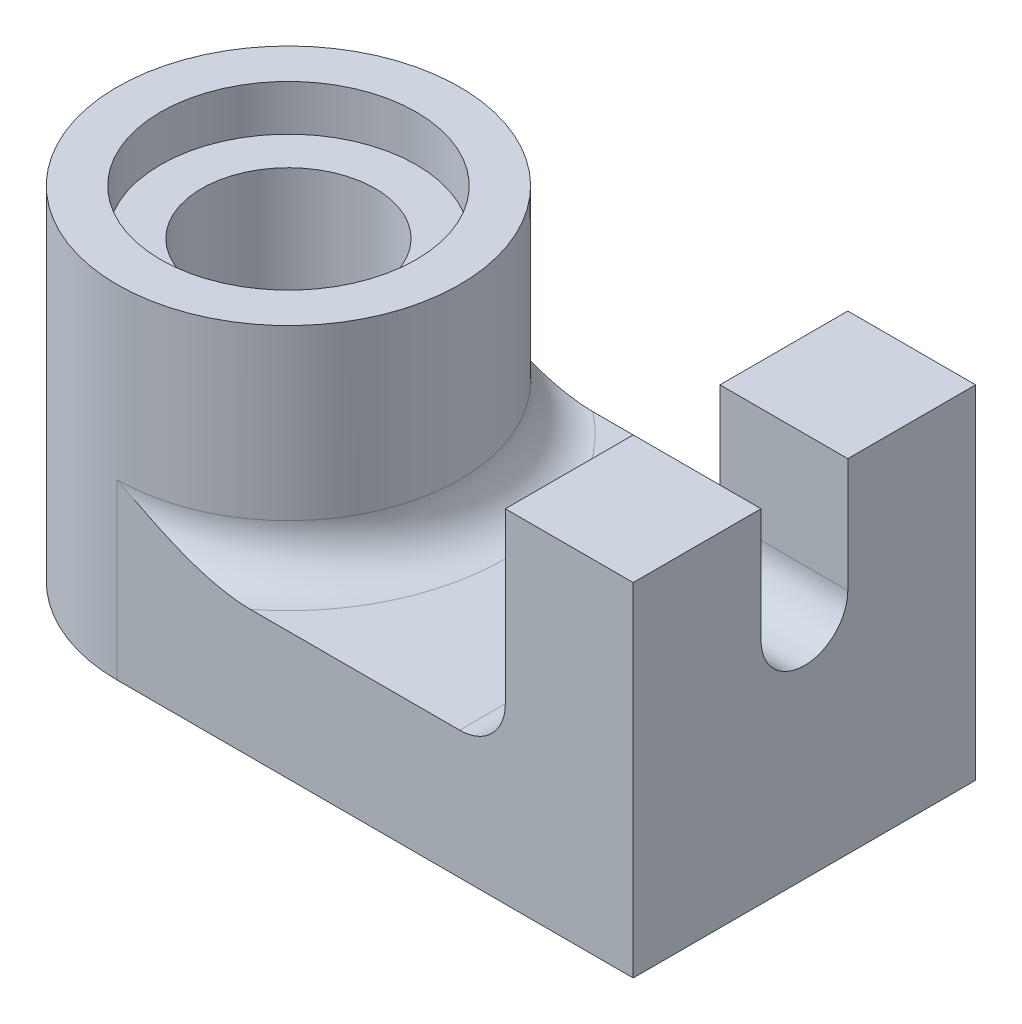
ISO-10303-21;
HEADER;
FILE_DESCRIPTION(('STEP AP214'),'2;1');
FILE_NAME('part.step','',(''),(''),'','','');
FILE_SCHEMA(('AUTOMOTIVE_DESIGN { 1 0 10303 214 1 1 1 1 }'));
ENDSEC;
DATA;
#1=APPLICATION_CONTEXT('core data for automotive mechanical design processes');
#2=APPLICATION_PROTOCOL_DEFINITION('international standard','automotive_design',2000,#1);
#3=PRODUCT_CONTEXT('',#1,'mechanical');
#4=PRODUCT('Part','Part','',(#3));
#5=PRODUCT_RELATED_PRODUCT_CATEGORY('part','',(#4));
#6=PRODUCT_DEFINITION_FORMATION('','',#4);
#7=PRODUCT_DEFINITION_CONTEXT('part definition',#1,'design');
#8=PRODUCT_DEFINITION('design','',#6,#7);
#9=PRODUCT_DEFINITION_SHAPE('','',#8);
#10=(LENGTH_UNIT() NAMED_UNIT(*) SI_UNIT(.MILLI.,.METRE.));
#11=(NAMED_UNIT(*) PLANE_ANGLE_UNIT() SI_UNIT($,.RADIAN.));
#12=(NAMED_UNIT(*) SI_UNIT($,.STERADIAN.) SOLID_ANGLE_UNIT());
#13=UNCERTAINTY_MEASURE_WITH_UNIT(LENGTH_MEASURE(1.E-05),#10,'distance_accuracy_value','');
#14=(GEOMETRIC_REPRESENTATION_CONTEXT(3) GLOBAL_UNCERTAINTY_ASSIGNED_CONTEXT((#13)) GLOBAL_UNIT_ASSIGNED_CONTEXT((#10,
#11,#12)) REPRESENTATION_CONTEXT('',''));
#15=CARTESIAN_POINT('',(0.,0.,0.));
#16=DIRECTION('',(0.,0.,1.));
#17=DIRECTION('',(1.,0.,0.));
#18=AXIS2_PLACEMENT_3D('',#15,#16,#17);
#19=CARTESIAN_POINT('',(0.,75.,0.));
#20=DIRECTION('',(0.,-1.,0.));
#21=DIRECTION('',(0.,0.,-1.));
#22=AXIS2_PLACEMENT_3D('',#19,#20,#21);
#23=PLANE('',#22);
#24=DIRECTION('',(0.,0.,-1.));
#25=VECTOR('',#24,1.);
#26=CARTESIAN_POINT('',(113.,75.,-37.5));
#27=LINE('',#26,#25);
#28=CARTESIAN_POINT('',(113.,75.,37.5));
#29=VERTEX_POINT('',#28);
#30=CARTESIAN_POINT('',(113.,75.,9.49999999999999));
#31=VERTEX_POINT('',#30);
#32=EDGE_CURVE('E204',#29,#31,#27,.T.);
#33=ORIENTED_EDGE('',*,*,#32,.T.);
#34=DIRECTION('',(-1.,0.,0.));
#35=VECTOR('',#34,1.);
#36=CARTESIAN_POINT('',(0.,75.,9.49999999999999));
#37=LINE('',#36,#35);
#38=CARTESIAN_POINT('',(85.,75.,9.49999999999999));
#39=VERTEX_POINT('',#38);
#40=EDGE_CURVE('E267',#31,#39,#37,.T.);
#41=ORIENTED_EDGE('',*,*,#40,.T.);
#42=DIRECTION('',(0.,0.,1.));
#43=VECTOR('',#42,1.);
#44=CARTESIAN_POINT('',(85.,75.,37.5));
#45=LINE('',#44,#43);
#46=CARTESIAN_POINT('',(85.,75.,37.5));
#47=VERTEX_POINT('',#46);
#48=EDGE_CURVE('E207',#39,#47,#45,.T.);
#49=ORIENTED_EDGE('',*,*,#48,.T.);
#50=DIRECTION('',(1.,0.,0.));
#51=VECTOR('',#50,1.);
#52=CARTESIAN_POINT('',(113.,75.,37.5));
#53=LINE('',#52,#51);
#54=EDGE_CURVE('E213',#47,#29,#53,.T.);
#55=ORIENTED_EDGE('',*,*,#54,.T.);
#56=EDGE_LOOP('',(#33,#41,#49,#55));
#57=FACE_BOUND('',#56,.T.);
#58=ADVANCED_FACE('F44',(#57),#23,.F.);
#59=CARTESIAN_POINT('',(0.,28.,0.));
#60=DIRECTION('',(0.,-1.,0.));
#61=DIRECTION('',(0.,0.,-1.));
#62=AXIS2_PLACEMENT_3D('',#59,#60,#61);
#63=PLANE('',#62);
#64=DIRECTION('',(-1.,0.,0.));
#65=VECTOR('',#64,1.);
#66=CARTESIAN_POINT('',(0.,28.,37.5));
#67=LINE('',#66,#65);
#68=CARTESIAN_POINT('',(75.,28.,37.5));
#69=VERTEX_POINT('',#68);
#70=CARTESIAN_POINT('',(29.1547594742265,28.,37.5));
#71=VERTEX_POINT('',#70);
#72=EDGE_CURVE('E223',#69,#71,#67,.T.);
#73=ORIENTED_EDGE('',*,*,#72,.F.);
#74=DIRECTION('',(0.,0.,1.));
#75=VECTOR('',#74,1.);
#76=CARTESIAN_POINT('',(75.,28.,-37.5));
#77=LINE('',#76,#75);
#78=CARTESIAN_POINT('',(75.,28.,-37.5));
#79=VERTEX_POINT('',#78);
#80=EDGE_CURVE('E386',#69,#79,#77,.F.);
#81=ORIENTED_EDGE('',*,*,#80,.T.);
#82=DIRECTION('',(1.,0.,0.));
#83=VECTOR('',#82,1.);
#84=CARTESIAN_POINT('',(113.,28.,-37.5));
#85=LINE('',#84,#83);
#86=CARTESIAN_POINT('',(29.1547594742265,28.,-37.5));
#87=VERTEX_POINT('',#86);
#88=EDGE_CURVE('E225',#87,#79,#85,.T.);
#89=ORIENTED_EDGE('',*,*,#88,.F.);
#90=CARTESIAN_POINT('',(0.,28.,0.));
#91=DIRECTION('',(0.,-1.,0.));
#92=DIRECTION('',(0.,0.,-1.));
#93=AXIS2_PLACEMENT_3D('',#90,#91,#92);
#94=CIRCLE('',#93,47.5);
#95=EDGE_CURVE('E279',#87,#71,#94,.T.);
#96=ORIENTED_EDGE('',*,*,#95,.T.);
#97=EDGE_LOOP('',(#73,#81,#89,#96));
#98=FACE_BOUND('',#97,.T.);
#99=ADVANCED_FACE('F309',(#98),#63,.F.);
#100=CARTESIAN_POINT('',(0.,75.,0.));
#101=DIRECTION('',(0.,-1.,0.));
#102=DIRECTION('',(0.,0.,-1.));
#103=AXIS2_PLACEMENT_3D('',#100,#101,#102);
#104=CYLINDRICAL_SURFACE('',#103,37.5);
#105=CARTESIAN_POINT('',(0.,75.,0.));
#106=DIRECTION('',(0.,1.,0.));
#107=DIRECTION('',(0.,0.,1.));
#108=AXIS2_PLACEMENT_3D('',#105,#106,#107);
#109=CIRCLE('',#108,37.5);
#110=CARTESIAN_POINT('',(0.,75.,37.5));
#111=VERTEX_POINT('',#110);
#112=EDGE_CURVE('E261',#111,#111,#109,.T.);
#113=ORIENTED_EDGE('',*,*,#112,.F.);
#114=EDGE_LOOP('',(#113));
#115=FACE_BOUND('',#114,.T.);
#116=CARTESIAN_POINT('',(0.,38.,0.));
#117=DIRECTION('',(0.,-1.,0.));
#118=DIRECTION('',(0.,0.,-1.));
#119=AXIS2_PLACEMENT_3D('',#116,#117,#118);
#120=CIRCLE('',#119,37.5);
#121=CARTESIAN_POINT('',(0.,38.,37.5));
#122=VERTEX_POINT('',#121);
#123=CARTESIAN_POINT('',(0.,38.,-37.5));
#124=VERTEX_POINT('',#123);
#125=EDGE_CURVE('E274',#122,#124,#120,.F.);
#126=ORIENTED_EDGE('',*,*,#125,.T.);
#127=DIRECTION('',(0.,-1.,0.));
#128=VECTOR('',#127,1.);
#129=CARTESIAN_POINT('',(0.,28.,-37.5));
#130=LINE('',#129,#128);
#131=CARTESIAN_POINT('',(0.,0.,-37.5));
#132=VERTEX_POINT('',#131);
#133=EDGE_CURVE('E230',#124,#132,#130,.T.);
#134=ORIENTED_EDGE('',*,*,#133,.T.);
#135=CARTESIAN_POINT('',(0.,0.,0.));
#136=DIRECTION('',(0.,1.,0.));
#137=DIRECTION('',(0.,0.,1.));
#138=AXIS2_PLACEMENT_3D('',#135,#136,#137);
#139=CIRCLE('',#138,37.5);
#140=CARTESIAN_POINT('',(0.,0.,37.5));
#141=VERTEX_POINT('',#140);
#142=EDGE_CURVE('E256',#132,#141,#139,.T.);
#143=ORIENTED_EDGE('',*,*,#142,.T.);
#144=DIRECTION('',(0.,-1.,0.));
#145=VECTOR('',#144,1.);
#146=CARTESIAN_POINT('',(0.,28.,37.5));
#147=LINE('',#146,#145);
#148=EDGE_CURVE('E237',#122,#141,#147,.T.);
#149=ORIENTED_EDGE('',*,*,#148,.F.);
#150=EDGE_LOOP('',(#126,#134,#143,#149));
#151=FACE_BOUND('',#150,.T.);
#152=ADVANCED_FACE('F304',(#115,#151),#104,.T.);
#153=CARTESIAN_POINT('',(0.,75.,0.));
#154=DIRECTION('',(0.,1.,0.));
#155=DIRECTION('',(0.,0.,1.));
#156=AXIS2_PLACEMENT_3D('',#153,#154,#155);
#157=PLANE('',#156);
#158=CARTESIAN_POINT('',(0.,75.,0.));
#159=DIRECTION('',(0.,1.,0.));
#160=DIRECTION('',(0.,0.,1.));
#161=AXIS2_PLACEMENT_3D('',#158,#159,#160);
#162=CIRCLE('',#161,28.);
#163=CARTESIAN_POINT('',(0.,75.,28.));
#164=VERTEX_POINT('',#163);
#165=EDGE_CURVE('E253',#164,#164,#162,.T.);
#166=ORIENTED_EDGE('',*,*,#165,.F.);
#167=EDGE_LOOP('',(#166));
#168=FACE_BOUND('',#167,.T.);
#169=ORIENTED_EDGE('',*,*,#112,.T.);
#170=EDGE_LOOP('',(#169));
#171=FACE_BOUND('',#170,.T.);
#172=ADVANCED_FACE('F310',(#168,#171),#157,.T.);
#173=CARTESIAN_POINT('',(0.,0.,0.));
#174=DIRECTION('',(0.,1.,0.));
#175=DIRECTION('',(0.,0.,1.));
#176=AXIS2_PLACEMENT_3D('',#173,#174,#175);
#177=PLANE('',#176);
#178=CARTESIAN_POINT('',(0.,0.,0.));
#179=DIRECTION('',(0.,-1.,0.));
#180=DIRECTION('',(0.,0.,-1.));
#181=AXIS2_PLACEMENT_3D('',#178,#179,#180);
#182=CIRCLE('',#181,28.);
#183=CARTESIAN_POINT('',(0.,0.,-28.));
#184=VERTEX_POINT('',#183);
#185=EDGE_CURVE('E252',#184,#184,#182,.T.);
#186=ORIENTED_EDGE('',*,*,#185,.F.);
#187=EDGE_LOOP('',(#186));
#188=FACE_BOUND('',#187,.T.);
#189=ORIENTED_EDGE('',*,*,#142,.F.);
#190=DIRECTION('',(1.,0.,0.));
#191=VECTOR('',#190,1.);
#192=CARTESIAN_POINT('',(113.,0.,-37.5));
#193=LINE('',#192,#191);
#194=CARTESIAN_POINT('',(113.,0.,-37.5));
#195=VERTEX_POINT('',#194);
#196=EDGE_CURVE('E222',#132,#195,#193,.T.);
#197=ORIENTED_EDGE('',*,*,#196,.T.);
#198=DIRECTION('',(0.,0.,1.));
#199=VECTOR('',#198,1.);
#200=CARTESIAN_POINT('',(113.,0.,37.5));
#201=LINE('',#200,#199);
#202=CARTESIAN_POINT('',(113.,0.,37.5));
#203=VERTEX_POINT('',#202);
#204=EDGE_CURVE('E231',#195,#203,#201,.T.);
#205=ORIENTED_EDGE('',*,*,#204,.T.);
#206=DIRECTION('',(-1.,0.,0.));
#207=VECTOR('',#206,1.);
#208=CARTESIAN_POINT('',(0.,0.,37.5));
#209=LINE('',#208,#207);
#210=EDGE_CURVE('E227',#203,#141,#209,.T.);
#211=ORIENTED_EDGE('',*,*,#210,.T.);
#212=EDGE_LOOP('',(#189,#197,#205,#211));
#213=FACE_BOUND('',#212,.T.);
#214=ADVANCED_FACE('F315',(#188,#213),#177,.F.);
#215=CARTESIAN_POINT('',(0.,65.,0.));
#216=DIRECTION('',(0.,1.,0.));
#217=DIRECTION('',(0.,0.,1.));
#218=AXIS2_PLACEMENT_3D('',#215,#216,#217);
#219=CYLINDRICAL_SURFACE('',#218,28.);
#220=CARTESIAN_POINT('',(0.,65.,0.));
#221=DIRECTION('',(0.,1.,0.));
#222=DIRECTION('',(0.,0.,1.));
#223=AXIS2_PLACEMENT_3D('',#220,#221,#222);
#224=CIRCLE('',#223,28.);
#225=CARTESIAN_POINT('',(0.,65.,28.));
#226=VERTEX_POINT('',#225);
#227=EDGE_CURVE('E254',#226,#226,#224,.T.);
#228=ORIENTED_EDGE('',*,*,#227,.F.);
#229=EDGE_LOOP('',(#228));
#230=FACE_BOUND('',#229,.T.);
#231=ORIENTED_EDGE('',*,*,#165,.T.);
#232=EDGE_LOOP('',(#231));
#233=FACE_BOUND('',#232,.T.);
#234=ADVANCED_FACE('F312',(#230,#233),#219,.F.);
#235=CARTESIAN_POINT('',(0.,65.,0.));
#236=DIRECTION('',(0.,1.,0.));
#237=DIRECTION('',(0.,0.,1.));
#238=AXIS2_PLACEMENT_3D('',#235,#236,#237);
#239=PLANE('',#238);
#240=DIRECTION('',(1.,0.,0.));
#241=VECTOR('',#240,1.);
#242=CARTESIAN_POINT('',(11.8084018470041,65.,5.));
#243=LINE('',#242,#241);
#244=CARTESIAN_POINT('',(18.3303027798234,65.,5.));
#245=VERTEX_POINT('',#244);
#246=CARTESIAN_POINT('',(22.,65.,5.));
#247=VERTEX_POINT('',#246);
#248=EDGE_CURVE('E162',#245,#247,#243,.T.);
#249=ORIENTED_EDGE('',*,*,#248,.F.);
#250=CARTESIAN_POINT('',(0.,65.,0.));
#251=DIRECTION('',(0.,1.,0.));
#252=DIRECTION('',(0.,0.,1.));
#253=AXIS2_PLACEMENT_3D('',#250,#251,#252);
#254=CIRCLE('',#253,19.);
#255=CARTESIAN_POINT('',(18.3303027798234,65.,-5.));
#256=VERTEX_POINT('',#255);
#257=EDGE_CURVE('E180',#256,#245,#254,.T.);
#258=ORIENTED_EDGE('',*,*,#257,.F.);
#259=DIRECTION('',(-1.,0.,0.));
#260=VECTOR('',#259,1.);
#261=CARTESIAN_POINT('',(22.,65.,-5.));
#262=LINE('',#261,#260);
#263=CARTESIAN_POINT('',(22.,65.,-5.));
#264=VERTEX_POINT('',#263);
#265=EDGE_CURVE('E58',#264,#256,#262,.T.);
#266=ORIENTED_EDGE('',*,*,#265,.F.);
#267=DIRECTION('',(0.,0.,-1.));
#268=VECTOR('',#267,1.);
#269=CARTESIAN_POINT('',(22.,65.,0.));
#270=LINE('',#269,#268);
#271=EDGE_CURVE('E167',#247,#264,#270,.T.);
#272=ORIENTED_EDGE('',*,*,#271,.F.);
#273=EDGE_LOOP('',(#249,#258,#266,#272));
#274=FACE_BOUND('',#273,.T.);
#275=ORIENTED_EDGE('',*,*,#227,.T.);
#276=EDGE_LOOP('',(#275));
#277=FACE_BOUND('',#276,.T.);
#278=ADVANCED_FACE('F171',(#274,#277),#239,.T.);
#279=CARTESIAN_POINT('',(0.,10.,0.));
#280=DIRECTION('',(0.,-1.,0.));
#281=DIRECTION('',(0.,0.,-1.));
#282=AXIS2_PLACEMENT_3D('',#279,#280,#281);
#283=CYLINDRICAL_SURFACE('',#282,28.);
#284=CARTESIAN_POINT('',(0.,10.,0.));
#285=DIRECTION('',(0.,-1.,0.));
#286=DIRECTION('',(0.,0.,-1.));
#287=AXIS2_PLACEMENT_3D('',#284,#285,#286);
#288=CIRCLE('',#287,28.);
#289=CARTESIAN_POINT('',(0.,10.,-28.));
#290=VERTEX_POINT('',#289);
#291=EDGE_CURVE('E247',#290,#290,#288,.T.);
#292=ORIENTED_EDGE('',*,*,#291,.F.);
#293=EDGE_LOOP('',(#292));
#294=FACE_BOUND('',#293,.T.);
#295=ORIENTED_EDGE('',*,*,#185,.T.);
#296=EDGE_LOOP('',(#295));
#297=FACE_BOUND('',#296,.T.);
#298=ADVANCED_FACE('F324',(#294,#297),#283,.F.);
#299=CARTESIAN_POINT('',(0.,10.,0.));
#300=DIRECTION('',(0.,-1.,0.));
#301=DIRECTION('',(0.,0.,-1.));
#302=AXIS2_PLACEMENT_3D('',#299,#300,#301);
#303=PLANE('',#302);
#304=DIRECTION('',(-1.,0.,0.));
#305=VECTOR('',#304,1.);
#306=CARTESIAN_POINT('',(0.,10.,5.));
#307=LINE('',#306,#305);
#308=CARTESIAN_POINT('',(22.,10.,5.));
#309=VERTEX_POINT('',#308);
#310=CARTESIAN_POINT('',(18.3303027798234,9.99999999999995,5.));
#311=VERTEX_POINT('',#310);
#312=EDGE_CURVE('E181',#309,#311,#307,.T.);
#313=ORIENTED_EDGE('',*,*,#312,.F.);
#314=DIRECTION('',(0.,0.,1.));
#315=VECTOR('',#314,1.);
#316=CARTESIAN_POINT('',(22.,10.,0.));
#317=LINE('',#316,#315);
#318=CARTESIAN_POINT('',(22.,10.,-5.));
#319=VERTEX_POINT('',#318);
#320=EDGE_CURVE('E11',#319,#309,#317,.T.);
#321=ORIENTED_EDGE('',*,*,#320,.F.);
#322=DIRECTION('',(1.,0.,0.));
#323=VECTOR('',#322,1.);
#324=CARTESIAN_POINT('',(0.,10.,-5.));
#325=LINE('',#324,#323);
#326=CARTESIAN_POINT('',(18.3303027798234,9.99999999999995,-5.));
#327=VERTEX_POINT('',#326);
#328=EDGE_CURVE('E157',#327,#319,#325,.T.);
#329=ORIENTED_EDGE('',*,*,#328,.F.);
#330=CARTESIAN_POINT('',(0.,10.,0.));
#331=DIRECTION('',(0.,-1.,0.));
#332=DIRECTION('',(0.,0.,-1.));
#333=AXIS2_PLACEMENT_3D('',#330,#331,#332);
#334=CIRCLE('',#333,19.);
#335=EDGE_CURVE('E239',#311,#327,#334,.T.);
#336=ORIENTED_EDGE('',*,*,#335,.F.);
#337=EDGE_LOOP('',(#313,#321,#329,#336));
#338=FACE_BOUND('',#337,.T.);
#339=ORIENTED_EDGE('',*,*,#291,.T.);
#340=EDGE_LOOP('',(#339));
#341=FACE_BOUND('',#340,.T.);
#342=ADVANCED_FACE('F327',(#338,#341),#303,.T.);
#343=CARTESIAN_POINT('',(0.,294.,0.));
#344=DIRECTION('',(0.,-1.,0.));
#345=DIRECTION('',(0.,0.,-1.));
#346=AXIS2_PLACEMENT_3D('',#343,#344,#345);
#347=CYLINDRICAL_SURFACE('',#346,19.);
#348=ORIENTED_EDGE('',*,*,#257,.T.);
#349=DIRECTION('',(0.,-1.,0.));
#350=VECTOR('',#349,1.);
#351=CARTESIAN_POINT('',(18.3303027798234,294.,5.));
#352=LINE('',#351,#350);
#353=EDGE_CURVE('E52',#245,#311,#352,.T.);
#354=ORIENTED_EDGE('',*,*,#353,.T.);
#355=ORIENTED_EDGE('',*,*,#335,.T.);
#356=DIRECTION('',(0.,-1.,0.));
#357=VECTOR('',#356,1.);
#358=CARTESIAN_POINT('',(18.3303027798234,294.,-5.));
#359=LINE('',#358,#357);
#360=EDGE_CURVE('E387',#327,#256,#359,.F.);
#361=ORIENTED_EDGE('',*,*,#360,.T.);
#362=EDGE_LOOP('',(#348,#354,#355,#361));
#363=FACE_BOUND('',#362,.T.);
#364=ADVANCED_FACE('F332',(#363),#347,.F.);
#365=CARTESIAN_POINT('',(0.,28.,37.5));
#366=DIRECTION('',(0.,0.,1.));
#367=DIRECTION('',(1.,0.,0.));
#368=AXIS2_PLACEMENT_3D('',#365,#366,#367);
#369=PLANE('',#368);
#370=ORIENTED_EDGE('',*,*,#210,.F.);
#371=DIRECTION('',(0.,-1.,0.));
#372=VECTOR('',#371,1.);
#373=CARTESIAN_POINT('',(113.,28.,37.5));
#374=LINE('',#373,#372);
#375=EDGE_CURVE('E238',#29,#203,#374,.T.);
#376=ORIENTED_EDGE('',*,*,#375,.F.);
#377=ORIENTED_EDGE('',*,*,#54,.F.);
#378=DIRECTION('',(0.,-1.,0.));
#379=VECTOR('',#378,1.);
#380=CARTESIAN_POINT('',(85.,75.,37.5));
#381=LINE('',#380,#379);
#382=CARTESIAN_POINT('',(85.,38.,37.5));
#383=VERTEX_POINT('',#382);
#384=EDGE_CURVE('E216',#47,#383,#381,.T.);
#385=ORIENTED_EDGE('',*,*,#384,.T.);
#386=CARTESIAN_POINT('',(75.,38.,37.5));
#387=DIRECTION('',(0.,0.,1.));
#388=DIRECTION('',(1.,0.,0.));
#389=AXIS2_PLACEMENT_3D('',#386,#387,#388);
#390=CIRCLE('',#389,10.);
#391=EDGE_CURVE('E67',#383,#69,#390,.F.);
#392=ORIENTED_EDGE('',*,*,#391,.T.);
#393=ORIENTED_EDGE('',*,*,#72,.T.);
#394=CARTESIAN_POINT('',(29.1547594742265,28.,37.5));
#395=CARTESIAN_POINT('',(28.7281693213262,28.0000213351898,37.5));
#396=CARTESIAN_POINT('',(28.3016560020065,28.0102823714574,37.5));
#397=CARTESIAN_POINT('',(27.4496484749399,28.0497436177248,37.5));
#398=CARTESIAN_POINT('',(27.0241539567352,28.0789370387632,37.5));
#399=CARTESIAN_POINT('',(26.1755938350896,28.1546490977663,37.5));
#400=CARTESIAN_POINT('',(25.7525250728232,28.2011328969961,37.5));
#401=CARTESIAN_POINT('',(24.9084309648025,28.3100570735608,37.5));
#402=CARTESIAN_POINT('',(24.4874058253523,28.3724990290878,37.5));
#403=CARTESIAN_POINT('',(23.2383730962953,28.5800893016702,37.5));
#404=CARTESIAN_POINT('',(22.4138500474495,28.7465122101732,37.5));
#405=CARTESIAN_POINT('',(20.7758132686323,29.1277255658412,37.5));
#406=CARTESIAN_POINT('',(19.9623061865978,29.3425439504518,37.5));
#407=CARTESIAN_POINT('',(18.3204624353024,29.8206084774631,37.5));
#408=CARTESIAN_POINT('',(17.4925271858517,30.0852230909812,37.5));
#409=CARTESIAN_POINT('',(15.8489631392484,30.6504595312053,37.5));
#410=CARTESIAN_POINT('',(15.0333369587737,30.9510888958736,37.5));
#411=CARTESIAN_POINT('',(13.4132111825217,31.5819324738925,37.5));
#412=CARTESIAN_POINT('',(12.6087174047981,31.9121615291726,37.5));
#413=CARTESIAN_POINT('',(11.0098130339229,32.5962759351171,37.5));
#414=CARTESIAN_POINT('',(10.2154035091012,32.9501637677222,37.5));
#415=CARTESIAN_POINT('',(7.83689487855474,34.0428931216893,37.5));
#416=CARTESIAN_POINT('',(6.26563680594967,34.8095165086093,37.5));
#417=CARTESIAN_POINT('',(3.14103857072318,36.3781249222061,37.5));
#418=CARTESIAN_POINT('',(1.5877013480228,37.1801156496955,37.5));
#419=CARTESIAN_POINT('',(0.0229415743836057,37.9881530227523,37.5));
#420=CARTESIAN_POINT('',(0.0114707876968247,37.9940765115417,37.5));
#421=CARTESIAN_POINT('',(0.,38.,37.5));
#422=B_SPLINE_CURVE_WITH_KNOTS('',3,(#394,#395,#396,#397,#398,#399,#400,#401,#402,#403,#404,
#405,#406,#407,#408,#409,#410,#411,#412,#413,#414,#415,#416,#417,#418,#419,#420,#421),
.UNSPECIFIED.,.F.,.F.,(4,2,2,2,2,2,2,2,2,2,2,2,2,4),(0.,1.27953571375756,2.5586128524898,
3.83512659165023,5.11176662134154,7.6333015052671,10.156295752437,12.7628652516246,
15.3699812675363,17.9784119404053,20.5871166832299,25.8307743780488,31.0752804024472,
31.1140102359087),.UNSPECIFIED.);
#423=EDGE_CURVE('E287',#71,#122,#422,.T.);
#424=ORIENTED_EDGE('',*,*,#423,.T.);
#425=ORIENTED_EDGE('',*,*,#148,.T.);
#426=EDGE_LOOP('',(#370,#376,#377,#385,#392,#393,#424,#425));
#427=FACE_BOUND('',#426,.T.);
#428=ADVANCED_FACE('F331',(#427),#369,.T.);
#429=CARTESIAN_POINT('',(113.,28.,37.5));
#430=DIRECTION('',(1.,0.,0.));
#431=DIRECTION('',(0.,0.,-1.));
#432=AXIS2_PLACEMENT_3D('',#429,#430,#431);
#433=PLANE('',#432);
#434=DIRECTION('',(0.,-1.,0.));
#435=VECTOR('',#434,1.);
#436=CARTESIAN_POINT('',(113.,50.,9.5));
#437=LINE('',#436,#435);
#438=CARTESIAN_POINT('',(113.,50.,9.5));
#439=VERTEX_POINT('',#438);
#440=EDGE_CURVE('E188',#31,#439,#437,.T.);
#441=ORIENTED_EDGE('',*,*,#440,.F.);
#442=ORIENTED_EDGE('',*,*,#32,.F.);
#443=ORIENTED_EDGE('',*,*,#375,.T.);
#444=ORIENTED_EDGE('',*,*,#204,.F.);
#445=DIRECTION('',(0.,-1.,0.));
#446=VECTOR('',#445,1.);
#447=CARTESIAN_POINT('',(113.,28.,-37.5));
#448=LINE('',#447,#446);
#449=CARTESIAN_POINT('',(113.,75.,-37.5));
#450=VERTEX_POINT('',#449);
#451=EDGE_CURVE('E244',#450,#195,#448,.T.);
#452=ORIENTED_EDGE('',*,*,#451,.F.);
#453=CARTESIAN_POINT('',(113.,75.,-9.5));
#454=VERTEX_POINT('',#453);
#455=EDGE_CURVE('E201',#454,#450,#27,.T.);
#456=ORIENTED_EDGE('',*,*,#455,.F.);
#457=DIRECTION('',(0.,1.,0.));
#458=VECTOR('',#457,1.);
#459=CARTESIAN_POINT('',(113.,50.,-9.5));
#460=LINE('',#459,#458);
#461=CARTESIAN_POINT('',(113.,50.,-9.5));
#462=VERTEX_POINT('',#461);
#463=EDGE_CURVE('E190',#462,#454,#460,.T.);
#464=ORIENTED_EDGE('',*,*,#463,.F.);
#465=CARTESIAN_POINT('',(113.,50.,0.));
#466=DIRECTION('',(1.,0.,0.));
#467=DIRECTION('',(0.,0.,-1.));
#468=AXIS2_PLACEMENT_3D('',#465,#466,#467);
#469=CIRCLE('',#468,9.5);
#470=EDGE_CURVE('E183',#439,#462,#469,.T.);
#471=ORIENTED_EDGE('',*,*,#470,.F.);
#472=EDGE_LOOP('',(#441,#442,#443,#444,#452,#456,#464,#471));
#473=FACE_BOUND('',#472,.T.);
#474=ADVANCED_FACE('F338',(#473),#433,.T.);
#475=CARTESIAN_POINT('',(113.,28.,-37.5));
#476=DIRECTION('',(0.,0.,-1.));
#477=DIRECTION('',(-1.,0.,0.));
#478=AXIS2_PLACEMENT_3D('',#475,#476,#477);
#479=PLANE('',#478);
#480=ORIENTED_EDGE('',*,*,#196,.F.);
#481=ORIENTED_EDGE('',*,*,#133,.F.);
#482=CARTESIAN_POINT('',(29.1547594742265,28.,-37.5));
#483=CARTESIAN_POINT('',(28.7281693213262,28.0000213351898,-37.5));
#484=CARTESIAN_POINT('',(28.3016560020065,28.0102823714574,-37.5));
#485=CARTESIAN_POINT('',(27.4496484749399,28.0497436177248,-37.5));
#486=CARTESIAN_POINT('',(27.0241539567352,28.0789370387632,-37.5));
#487=CARTESIAN_POINT('',(26.1755938350896,28.1546490977663,-37.5));
#488=CARTESIAN_POINT('',(25.7525250728232,28.2011328969961,-37.5));
#489=CARTESIAN_POINT('',(24.9084309648025,28.3100570735608,-37.5));
#490=CARTESIAN_POINT('',(24.4874058253523,28.3724990290878,-37.5));
#491=CARTESIAN_POINT('',(23.2383730962953,28.5800893016702,-37.5));
#492=CARTESIAN_POINT('',(22.4138500474495,28.7465122101732,-37.5));
#493=CARTESIAN_POINT('',(20.7758132686323,29.1277255658412,-37.5));
#494=CARTESIAN_POINT('',(19.9623061865978,29.3425439504518,-37.5));
#495=CARTESIAN_POINT('',(18.3204624353024,29.8206084774631,-37.5));
#496=CARTESIAN_POINT('',(17.4925271858517,30.0852230909812,-37.5));
#497=CARTESIAN_POINT('',(15.8489631392484,30.6504595312053,-37.5));
#498=CARTESIAN_POINT('',(15.0333369587737,30.9510888958736,-37.5));
#499=CARTESIAN_POINT('',(13.4132111825217,31.5819324738925,-37.5));
#500=CARTESIAN_POINT('',(12.6087174047981,31.9121615291726,-37.5));
#501=CARTESIAN_POINT('',(11.0098130339229,32.5962759351171,-37.5));
#502=CARTESIAN_POINT('',(10.2154035091012,32.9501637677222,-37.5));
#503=CARTESIAN_POINT('',(7.83689487855474,34.0428931216893,-37.5));
#504=CARTESIAN_POINT('',(6.26563680594967,34.8095165086093,-37.5));
#505=CARTESIAN_POINT('',(3.14103857072318,36.3781249222061,-37.5));
#506=CARTESIAN_POINT('',(1.5877013480228,37.1801156496955,-37.5));
#507=CARTESIAN_POINT('',(0.0229415743836057,37.9881530227523,-37.5));
#508=CARTESIAN_POINT('',(0.0114707876968247,37.9940765115417,-37.5));
#509=CARTESIAN_POINT('',(0.,38.,-37.5));
#510=B_SPLINE_CURVE_WITH_KNOTS('',3,(#482,#483,#484,#485,#486,#487,#488,#489,#490,#491,#492,
#493,#494,#495,#496,#497,#498,#499,#500,#501,#502,#503,#504,#505,#506,#507,#508,#509),
.UNSPECIFIED.,.F.,.F.,(4,2,2,2,2,2,2,2,2,2,2,2,2,4),(0.,1.27953571375756,2.5586128524898,
3.83512659165023,5.11176662134154,7.6333015052671,10.156295752437,12.7628652516246,
15.3699812675363,17.9784119404053,20.5871166832299,25.8307743780488,31.0752804024472,
31.1140102359087),.UNSPECIFIED.);
#511=EDGE_CURVE('E282',#124,#87,#510,.F.);
#512=ORIENTED_EDGE('',*,*,#511,.T.);
#513=ORIENTED_EDGE('',*,*,#88,.T.);
#514=CARTESIAN_POINT('',(75.,38.,-37.5));
#515=DIRECTION('',(0.,0.,-1.));
#516=DIRECTION('',(-1.,0.,0.));
#517=AXIS2_PLACEMENT_3D('',#514,#515,#516);
#518=CIRCLE('',#517,10.);
#519=CARTESIAN_POINT('',(85.,38.,-37.5));
#520=VERTEX_POINT('',#519);
#521=EDGE_CURVE('E385',#79,#520,#518,.F.);
#522=ORIENTED_EDGE('',*,*,#521,.T.);
#523=DIRECTION('',(0.,-1.,0.));
#524=VECTOR('',#523,1.);
#525=CARTESIAN_POINT('',(85.,75.,-37.5));
#526=LINE('',#525,#524);
#527=CARTESIAN_POINT('',(85.,75.,-37.5));
#528=VERTEX_POINT('',#527);
#529=EDGE_CURVE('E217',#528,#520,#526,.T.);
#530=ORIENTED_EDGE('',*,*,#529,.F.);
#531=DIRECTION('',(-1.,0.,0.));
#532=VECTOR('',#531,1.);
#533=CARTESIAN_POINT('',(85.,75.,-37.5));
#534=LINE('',#533,#532);
#535=EDGE_CURVE('E210',#450,#528,#534,.T.);
#536=ORIENTED_EDGE('',*,*,#535,.F.);
#537=ORIENTED_EDGE('',*,*,#451,.T.);
#538=EDGE_LOOP('',(#480,#481,#512,#513,#522,#530,#536,#537));
#539=FACE_BOUND('',#538,.T.);
#540=ADVANCED_FACE('F293',(#539),#479,.T.);
#541=CARTESIAN_POINT('',(85.,75.,37.5));
#542=DIRECTION('',(1.,0.,0.));
#543=DIRECTION('',(0.,0.,-1.));
#544=AXIS2_PLACEMENT_3D('',#541,#542,#543);
#545=PLANE('',#544);
#546=ORIENTED_EDGE('',*,*,#529,.T.);
#547=DIRECTION('',(0.,0.,1.));
#548=VECTOR('',#547,1.);
#549=CARTESIAN_POINT('',(85.,38.,37.5));
#550=LINE('',#549,#548);
#551=EDGE_CURVE('E617',#520,#383,#550,.T.);
#552=ORIENTED_EDGE('',*,*,#551,.T.);
#553=ORIENTED_EDGE('',*,*,#384,.F.);
#554=ORIENTED_EDGE('',*,*,#48,.F.);
#555=DIRECTION('',(0.,-1.,0.));
#556=VECTOR('',#555,1.);
#557=CARTESIAN_POINT('',(85.,75.,9.49999999999999));
#558=LINE('',#557,#556);
#559=CARTESIAN_POINT('',(85.,50.,9.5));
#560=VERTEX_POINT('',#559);
#561=EDGE_CURVE('E199',#39,#560,#558,.T.);
#562=ORIENTED_EDGE('',*,*,#561,.T.);
#563=CARTESIAN_POINT('',(85.,50.,0.));
#564=DIRECTION('',(1.,0.,0.));
#565=DIRECTION('',(0.,0.,-1.));
#566=AXIS2_PLACEMENT_3D('',#563,#564,#565);
#567=CIRCLE('',#566,9.5);
#568=CARTESIAN_POINT('',(85.,50.,-9.5));
#569=VERTEX_POINT('',#568);
#570=EDGE_CURVE('E275',#560,#569,#567,.T.);
#571=ORIENTED_EDGE('',*,*,#570,.T.);
#572=DIRECTION('',(0.,1.,0.));
#573=VECTOR('',#572,1.);
#574=CARTESIAN_POINT('',(85.,75.,-9.5));
#575=LINE('',#574,#573);
#576=CARTESIAN_POINT('',(85.,75.,-9.5));
#577=VERTEX_POINT('',#576);
#578=EDGE_CURVE('E198',#569,#577,#575,.T.);
#579=ORIENTED_EDGE('',*,*,#578,.T.);
#580=EDGE_CURVE('E209',#528,#577,#45,.T.);
#581=ORIENTED_EDGE('',*,*,#580,.F.);
#582=EDGE_LOOP('',(#546,#552,#553,#554,#562,#571,#579,#581));
#583=FACE_BOUND('',#582,.T.);
#584=ADVANCED_FACE('F353',(#583),#545,.F.);
#585=ORIENTED_EDGE('',*,*,#580,.T.);
#586=DIRECTION('',(1.,0.,0.));
#587=VECTOR('',#586,1.);
#588=CARTESIAN_POINT('',(0.,75.,-9.5));
#589=LINE('',#588,#587);
#590=EDGE_CURVE('E262',#577,#454,#589,.T.);
#591=ORIENTED_EDGE('',*,*,#590,.T.);
#592=ORIENTED_EDGE('',*,*,#455,.T.);
#593=ORIENTED_EDGE('',*,*,#535,.T.);
#594=EDGE_LOOP('',(#585,#591,#592,#593));
#595=FACE_BOUND('',#594,.T.);
#596=ADVANCED_FACE('F343',(#595),#23,.F.);
#597=CARTESIAN_POINT('',(66.,50.,0.));
#598=DIRECTION('',(1.,0.,0.));
#599=DIRECTION('',(0.,0.,-1.));
#600=AXIS2_PLACEMENT_3D('',#597,#598,#599);
#601=CYLINDRICAL_SURFACE('',#600,9.5);
#602=DIRECTION('',(1.,0.,0.));
#603=VECTOR('',#602,1.);
#604=CARTESIAN_POINT('',(66.,50.,9.5));
#605=LINE('',#604,#603);
#606=EDGE_CURVE('E193',#560,#439,#605,.T.);
#607=ORIENTED_EDGE('',*,*,#606,.T.);
#608=ORIENTED_EDGE('',*,*,#470,.T.);
#609=DIRECTION('',(1.,0.,0.));
#610=VECTOR('',#609,1.);
#611=CARTESIAN_POINT('',(66.,50.,-9.5));
#612=LINE('',#611,#610);
#613=EDGE_CURVE('E192',#569,#462,#612,.T.);
#614=ORIENTED_EDGE('',*,*,#613,.F.);
#615=ORIENTED_EDGE('',*,*,#570,.F.);
#616=EDGE_LOOP('',(#607,#608,#614,#615));
#617=FACE_BOUND('',#616,.T.);
#618=ADVANCED_FACE('F351',(#617),#601,.F.);
#619=CARTESIAN_POINT('',(66.,50.,9.5));
#620=DIRECTION('',(0.,0.,1.));
#621=DIRECTION('',(0.,-1.,0.));
#622=AXIS2_PLACEMENT_3D('',#619,#620,#621);
#623=PLANE('',#622);
#624=ORIENTED_EDGE('',*,*,#40,.F.);
#625=ORIENTED_EDGE('',*,*,#440,.T.);
#626=ORIENTED_EDGE('',*,*,#606,.F.);
#627=ORIENTED_EDGE('',*,*,#561,.F.);
#628=EDGE_LOOP('',(#624,#625,#626,#627));
#629=FACE_BOUND('',#628,.T.);
#630=ADVANCED_FACE('F359',(#629),#623,.F.);
#631=CARTESIAN_POINT('',(66.,50.,-9.5));
#632=DIRECTION('',(0.,0.,-1.));
#633=DIRECTION('',(0.,1.,0.));
#634=AXIS2_PLACEMENT_3D('',#631,#632,#633);
#635=PLANE('',#634);
#636=ORIENTED_EDGE('',*,*,#613,.T.);
#637=ORIENTED_EDGE('',*,*,#463,.T.);
#638=ORIENTED_EDGE('',*,*,#590,.F.);
#639=ORIENTED_EDGE('',*,*,#578,.F.);
#640=EDGE_LOOP('',(#636,#637,#638,#639));
#641=FACE_BOUND('',#640,.T.);
#642=ADVANCED_FACE('F302',(#641),#635,.F.);
#643=CARTESIAN_POINT('',(0.,38.,0.));
#644=DIRECTION('',(0.,-1.,0.));
#645=DIRECTION('',(0.,0.,-1.));
#646=AXIS2_PLACEMENT_3D('',#643,#644,#645);
#647=TOROIDAL_SURFACE('',#646,47.5,10.);
#648=ORIENTED_EDGE('',*,*,#423,.F.);
#649=ORIENTED_EDGE('',*,*,#95,.F.);
#650=ORIENTED_EDGE('',*,*,#511,.F.);
#651=ORIENTED_EDGE('',*,*,#125,.F.);
#652=EDGE_LOOP('',(#648,#649,#650,#651));
#653=FACE_BOUND('',#652,.T.);
#654=ADVANCED_FACE('F296',(#653),#647,.F.);
#655=CARTESIAN_POINT('',(75.,38.,37.5));
#656=DIRECTION('',(0.,0.,-1.));
#657=DIRECTION('',(-1.,0.,0.));
#658=AXIS2_PLACEMENT_3D('',#655,#656,#657);
#659=CYLINDRICAL_SURFACE('',#658,10.);
#660=ORIENTED_EDGE('',*,*,#521,.F.);
#661=ORIENTED_EDGE('',*,*,#80,.F.);
#662=ORIENTED_EDGE('',*,*,#391,.F.);
#663=ORIENTED_EDGE('',*,*,#551,.F.);
#664=EDGE_LOOP('',(#660,#661,#662,#663));
#665=FACE_BOUND('',#664,.T.);
#666=ADVANCED_FACE('F50',(#665),#659,.F.);
#667=CARTESIAN_POINT('',(11.8084018470041,-16.,5.));
#668=DIRECTION('',(0.,0.,1.));
#669=DIRECTION('',(1.,0.,0.));
#670=AXIS2_PLACEMENT_3D('',#667,#668,#669);
#671=PLANE('',#670);
#672=ORIENTED_EDGE('',*,*,#312,.T.);
#673=ORIENTED_EDGE('',*,*,#353,.F.);
#674=ORIENTED_EDGE('',*,*,#248,.T.);
#675=DIRECTION('',(0.,1.,0.));
#676=VECTOR('',#675,1.);
#677=CARTESIAN_POINT('',(22.,-16.,5.));
#678=LINE('',#677,#676);
#679=EDGE_CURVE('E165',#309,#247,#678,.T.);
#680=ORIENTED_EDGE('',*,*,#679,.F.);
#681=EDGE_LOOP('',(#672,#673,#674,#680));
#682=FACE_BOUND('',#681,.T.);
#683=ADVANCED_FACE('F400',(#682),#671,.F.);
#684=CARTESIAN_POINT('',(22.,-16.,-5.));
#685=DIRECTION('',(0.,0.,-1.));
#686=DIRECTION('',(-1.,0.,0.));
#687=AXIS2_PLACEMENT_3D('',#684,#685,#686);
#688=PLANE('',#687);
#689=ORIENTED_EDGE('',*,*,#328,.T.);
#690=DIRECTION('',(0.,1.,0.));
#691=VECTOR('',#690,1.);
#692=CARTESIAN_POINT('',(22.,-16.,-5.));
#693=LINE('',#692,#691);
#694=EDGE_CURVE('E154',#319,#264,#693,.T.);
#695=ORIENTED_EDGE('',*,*,#694,.T.);
#696=ORIENTED_EDGE('',*,*,#265,.T.);
#697=ORIENTED_EDGE('',*,*,#360,.F.);
#698=EDGE_LOOP('',(#689,#695,#696,#697));
#699=FACE_BOUND('',#698,.T.);
#700=ADVANCED_FACE('F160',(#699),#688,.F.);
#701=CARTESIAN_POINT('',(22.,-16.,0.));
#702=DIRECTION('',(1.,0.,0.));
#703=DIRECTION('',(0.,0.,-1.));
#704=AXIS2_PLACEMENT_3D('',#701,#702,#703);
#705=PLANE('',#704);
#706=ORIENTED_EDGE('',*,*,#320,.T.);
#707=ORIENTED_EDGE('',*,*,#679,.T.);
#708=ORIENTED_EDGE('',*,*,#271,.T.);
#709=ORIENTED_EDGE('',*,*,#694,.F.);
#710=EDGE_LOOP('',(#706,#707,#708,#709));
#711=FACE_BOUND('',#710,.T.);
#712=ADVANCED_FACE('F170',(#711),#705,.F.);
#713=CLOSED_SHELL('',(#58,#99,#152,#172,#214,#234,#278,#298,#342,#364,#428,#474,#540,#584,#596,
#618,#630,#642,#654,#666,#683,#700,#712));
#714=MANIFOLD_SOLID_BREP('B2',#713);
#715=ADVANCED_BREP_SHAPE_REPRESENTATION('',(#18,#714),#14);
#716=SHAPE_DEFINITION_REPRESENTATION(#9,#715);
ENDSEC;
END-ISO-10303-21;
